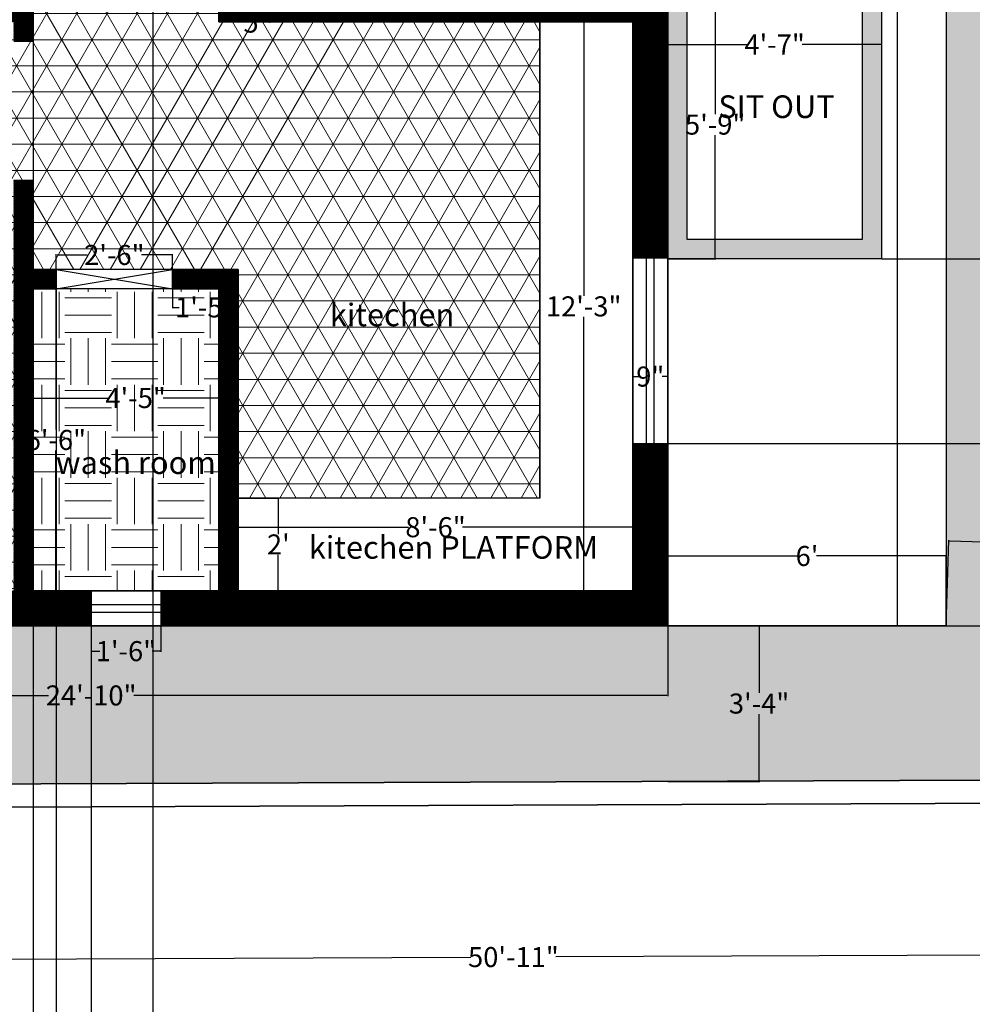
# Model space of a CAD drawing. Units: inches. Extents: x -157 to 1464, y -361 to 1077.
# Tile 4 of 9: x 430 to 676, y 14 to 268. Entities that reach past the tile are written whole.
import ezdxf

# ---------------------------------------------------------------- set-up
doc = ezdxf.new("R2010")
doc.units = ezdxf.units.IN
doc.header["$MEASUREMENT"] = 0
for name, color, linetype, lineweight in [('A-ANNO-DIMS', 2, 'Continuous', 18), ('A-ANNO-TEXT', 7, 'Continuous', 18), ('A-AREA-IDEN', 7, 'Continuous', 18), ('A-FLOR', 7, 'Continuous', 25), ('A-FLOR-FIXT', 9, 'Continuous', 25), ('A-FLOR-PATT', 8, 'Continuous', 13), ('A-WALL', 7, 'Continuous', 35), ('A-WALL-PATT', 252, 'Continuous', 13), ('C-ANNO-DIMS', 2, 'Continuous', 18), ('C-PROP', 7, 'Continuous', 35), ('doors and windows', 33, 'Continuous', 25), ('L-GRND-PATT', 8, 'Continuous', 13)]:
    doc.layers.add(name, color=color, linetype=linetype, lineweight=lineweight)
doc.styles.get("Standard").update_dxf_attribs({"font": 'arial.ttf'})
doc.dimstyles.new('Annotative', dxfattribs={"dimscale": 0, "dimtxt": 5.18, "dimasz": 0.18, "dimexe": 0.18, "dimexo": 0.0625, "dimgap": 0.09, "dimtad": 0, "dimtih": 1, "dimtoh": 1, "dimdec": 0, "dimzin": 0, "dimdsep": 46, "dimlunit": 3, "dimtxsty": 'Standard', "dimcen": 0.09, "dimadec": 0, "dimazin": 0, "dimtfac": 1, "dimtdec": 0, "dimtofl": 0, "dimtmove": 0, "dimatfit": 3, "dimfxl": 1, "dimtolj": 1, "dimtzin": 0, "dimarcsym": 0})

# ---------------------------------------------------------------- blocks, each defined once
blk = doc.blocks.new('*D2')
at = {"layer": 'A-ANNO-DIMS', "color": 0, "lineweight": -2, "transparency": 16777216}
for p, q in [((298.97, 111.8), (298.97, 93.67)), ((596.97, 111.8), (596.97, 93.67)), ((299.15, 93.85), (436.92, 93.85)), ((596.79, 93.85), (459.01, 93.85))]:
    blk.add_line(p, q, dxfattribs=at)
at = {"layer": 'A-ANNO-DIMS', "color": 0, "transparency": 16777216}
for points in [[(299.15, 93.88), (299.15, 93.82), (298.97, 93.85)], [(596.79, 93.88), (596.79, 93.82), (596.97, 93.85)]]:
    blk.add_solid(points, dxfattribs=at)
at = {"layer": 'Defpoints', "color": 0, "transparency": 16777216}
for p in [(298.97, 111.86), (596.97, 111.86), (596.97, 93.85)]:
    blk.add_point(p, dxfattribs=at)
at = {"layer": 'A-ANNO-DIMS', "color": 0, "transparency": 16777216, "insert": (447.97, 93.85), "char_height": 5.18, "attachment_point": 5}
blk.add_mtext('\\A1;24\'-10"', dxfattribs=at)
blk = doc.blocks.new('*D5')
at = {"layer": 'A-ANNO-DIMS', "color": 0, "lineweight": -2, "transparency": 16777216}
for p, q in [((433.03, 198.86), (439.03, 198.86)), ((438.85, 198.68), (438.85, 162.6)), ((438.85, 121.04), (438.85, 157.13)), ((433.03, 120.86), (439.03, 120.86))]:
    blk.add_line(p, q, dxfattribs=at)
at = {"layer": 'A-ANNO-DIMS', "color": 0, "transparency": 16777216}
for points in [[(438.82, 198.68), (438.88, 198.68), (438.85, 198.86)], [(438.82, 121.04), (438.88, 121.04), (438.85, 120.86)]]:
    blk.add_solid(points, dxfattribs=at)
at = {"layer": 'Defpoints', "color": 0, "transparency": 16777216}
for p in [(432.97, 198.86), (438.85, 198.86), (432.97, 120.86)]:
    blk.add_point(p, dxfattribs=at)
at = {"layer": 'A-ANNO-DIMS', "color": 0, "transparency": 16777216, "insert": (438.85, 159.86), "char_height": 5.18, "attachment_point": 5}
blk.add_mtext('\\A1;6\'-6"', dxfattribs=at)
blk = doc.blocks.new('*D6')
at = {"layer": 'A-ANNO-DIMS', "color": 0, "lineweight": -2, "transparency": 16777216}
for p, q in [((432.97, 198.8), (432.97, 170.51)), ((485.97, 198.8), (485.97, 170.51)), ((433.15, 170.69), (452.39, 170.69)), ((485.79, 170.69), (466.55, 170.69))]:
    blk.add_line(p, q, dxfattribs=at)
at = {"layer": 'A-ANNO-DIMS', "color": 0, "transparency": 16777216}
for points in [[(433.15, 170.72), (433.15, 170.66), (432.97, 170.69)], [(485.79, 170.72), (485.79, 170.66), (485.97, 170.69)]]:
    blk.add_solid(points, dxfattribs=at)
at = {"layer": 'Defpoints', "color": 0, "transparency": 16777216}
for p in [(432.97, 198.86), (485.97, 198.86), (485.97, 170.69)]:
    blk.add_point(p, dxfattribs=at)
at = {"layer": 'A-ANNO-DIMS', "color": 0, "transparency": 16777216, "insert": (459.47, 170.69), "char_height": 5.18, "attachment_point": 5}
blk.add_mtext('\\A1;4\'-5"', dxfattribs=at)
blk = doc.blocks.new('*D11')
at = {"layer": 'A-ANNO-DIMS', "color": 0, "lineweight": -2, "transparency": 16777216}
for p, q in [((485.97, 120.92), (485.97, 137.5)), ((587.97, 120.92), (587.97, 137.5)), ((486.15, 137.32), (529.99, 137.32)), ((587.79, 137.32), (543.95, 137.32))]:
    blk.add_line(p, q, dxfattribs=at)
at = {"layer": 'A-ANNO-DIMS', "color": 0, "transparency": 16777216}
for points in [[(486.15, 137.35), (486.15, 137.29), (485.97, 137.32)], [(587.79, 137.35), (587.79, 137.29), (587.97, 137.32)]]:
    blk.add_solid(points, dxfattribs=at)
at = {"layer": 'Defpoints', "color": 0, "transparency": 16777216}
for p in [(485.97, 137.32), (485.97, 120.86), (587.97, 120.86)]:
    blk.add_point(p, dxfattribs=at)
at = {"layer": 'A-ANNO-DIMS', "color": 0, "transparency": 16777216, "insert": (536.97, 137.32), "char_height": 5.18, "attachment_point": 5}
blk.add_mtext('\\A1;8\'-6"', dxfattribs=at)
blk = doc.blocks.new('*D12')
at = {"layer": 'A-ANNO-DIMS', "color": 0, "lineweight": -2, "transparency": 16777216}
for p, q in [((587.9, 267.86), (575.08, 267.86)), ((575.26, 267.68), (575.26, 197.1)), ((575.26, 121.04), (575.26, 191.62)), ((587.9, 120.86), (575.08, 120.86))]:
    blk.add_line(p, q, dxfattribs=at)
at = {"layer": 'A-ANNO-DIMS', "color": 0, "transparency": 16777216}
for points in [[(575.23, 267.68), (575.29, 267.68), (575.26, 267.86)], [(575.23, 121.04), (575.29, 121.04), (575.26, 120.86)]]:
    blk.add_solid(points, dxfattribs=at)
at = {"layer": 'Defpoints', "color": 0, "transparency": 16777216}
for p in [(575.26, 267.86), (587.97, 267.86), (587.97, 120.86)]:
    blk.add_point(p, dxfattribs=at)
at = {"layer": 'A-ANNO-DIMS', "color": 0, "transparency": 16777216, "insert": (575.26, 194.36), "char_height": 5.18, "attachment_point": 5}
blk.add_mtext('\\A1;12\'-3"', dxfattribs=at)
blk = doc.blocks.new('*D14')
at = {"layer": 'C-ANNO-DIMS', "color": 0, "lineweight": -2, "transparency": 16777216}
for p, q in [((862.57, 66.62), (862.72, 27.26)), ((251.33, 64.28), (251.48, 24.92)), ((251.66, 25.1), (546.1, 26.23)), ((862.54, 27.44), (568.1, 26.31))]:
    blk.add_line(p, q, dxfattribs=at)
at = {"layer": 'C-ANNO-DIMS', "color": 0, "transparency": 16777216}
for points in [[(862.54, 27.47), (862.54, 27.41), (862.72, 27.44)], [(251.66, 25.13), (251.66, 25.07), (251.48, 25.1)]]:
    blk.add_solid(points, dxfattribs=at)
at = {"layer": 'Defpoints', "color": 0, "transparency": 16777216}
for p in [(862.57, 66.68), (251.33, 64.34), (862.72, 27.44)]:
    blk.add_point(p, dxfattribs=at)
at = {"layer": 'C-ANNO-DIMS', "color": 0, "transparency": 16777216, "insert": (557.1, 26.27), "char_height": 5.18, "attachment_point": 5}
blk.add_mtext('\\A1;50\'-11"', dxfattribs=at)
blk = doc.blocks.new('*D22')
at = {"layer": 'A-ANNO-DIMS', "color": 0, "lineweight": -2, "transparency": 16777216}
for p, q in [((596.97, 111.92), (596.97, 130.06)), ((597.15, 129.88), (630.48, 129.88)), ((668.79, 129.88), (635.45, 129.88)), ((668.97, 111.92), (668.97, 130.06))]:
    blk.add_line(p, q, dxfattribs=at)
at = {"layer": 'A-ANNO-DIMS', "color": 0, "transparency": 16777216}
for points in [[(597.15, 129.91), (597.15, 129.85), (596.97, 129.88)], [(668.79, 129.91), (668.79, 129.85), (668.97, 129.88)]]:
    blk.add_solid(points, dxfattribs=at)
at = {"layer": 'Defpoints', "color": 0, "transparency": 16777216}
for p in [(596.97, 129.88), (596.97, 111.86), (668.97, 111.86)]:
    blk.add_point(p, dxfattribs=at)
at = {"layer": 'A-ANNO-DIMS', "color": 0, "transparency": 16777216, "insert": (632.97, 129.88), "char_height": 5.18, "attachment_point": 5}
blk.add_mtext("\\A1;6'", dxfattribs=at)
blk = doc.blocks.new('*D23')
at = {"layer": 'A-ANNO-DIMS', "color": 0, "lineweight": -2, "transparency": 16777216}
for p, q in [((668.9, 492.86), (656.18, 492.86)), ((656.36, 492.68), (656.36, 305.1)), ((656.36, 112.04), (656.36, 299.62)), ((668.9, 111.86), (656.18, 111.86))]:
    blk.add_line(p, q, dxfattribs=at)
at = {"layer": 'A-ANNO-DIMS', "color": 0, "transparency": 16777216}
for points in [[(656.33, 492.68), (656.39, 492.68), (656.36, 492.86)], [(656.33, 112.04), (656.39, 112.04), (656.36, 111.86)]]:
    blk.add_solid(points, dxfattribs=at)
at = {"layer": 'Defpoints', "color": 0, "transparency": 16777216}
for p in [(668.97, 492.86), (656.36, 111.86), (668.97, 111.86)]:
    blk.add_point(p, dxfattribs=at)
at = {"layer": 'A-ANNO-DIMS', "color": 0, "transparency": 16777216, "insert": (656.36, 302.36), "char_height": 5.18, "attachment_point": 5}
blk.add_mtext('\\A1;31\'-9"', dxfattribs=at)
blk = doc.blocks.new('*D26')
at = {"layer": 'A-ANNO-DIMS', "color": 0, "lineweight": -2, "transparency": 16777216}
for p, q in [((587.97, 184.35), (587.97, 176.05)), ((596.97, 184.35), (596.97, 176.05)), ((588.15, 176.23), (589.4, 176.23)), ((596.79, 176.23), (595.53, 176.23))]:
    blk.add_line(p, q, dxfattribs=at)
at = {"layer": 'A-ANNO-DIMS', "color": 0, "transparency": 16777216}
for points in [[(588.15, 176.26), (588.15, 176.2), (587.97, 176.23)], [(596.79, 176.26), (596.79, 176.2), (596.97, 176.23)]]:
    blk.add_solid(points, dxfattribs=at)
at = {"layer": 'Defpoints', "color": 0, "transparency": 16777216}
for p in [(587.97, 184.41), (596.97, 184.41), (596.97, 176.23)]:
    blk.add_point(p, dxfattribs=at)
at = {"layer": 'A-ANNO-DIMS', "color": 0, "transparency": 16777216, "insert": (592.47, 176.23), "char_height": 5.18, "attachment_point": 5}
blk.add_mtext('\\A1;9"', dxfattribs=at)
blk = doc.blocks.new('*D27')
at = {"layer": 'A-ANNO-DIMS', "color": 0, "lineweight": -2, "transparency": 16777216}
for p, q in [((486.03, 144.86), (496.52, 144.86)), ((496.34, 144.68), (496.34, 135.55)), ((496.34, 121.04), (496.34, 130.17)), ((486.03, 120.86), (496.52, 120.86))]:
    blk.add_line(p, q, dxfattribs=at)
at = {"layer": 'A-ANNO-DIMS', "color": 0, "transparency": 16777216}
for points in [[(496.31, 144.68), (496.37, 144.68), (496.34, 144.86)], [(496.31, 121.04), (496.37, 121.04), (496.34, 120.86)]]:
    blk.add_solid(points, dxfattribs=at)
at = {"layer": 'Defpoints', "color": 0, "transparency": 16777216}
for p in [(485.97, 144.86), (485.97, 120.86), (496.34, 120.86)]:
    blk.add_point(p, dxfattribs=at)
at = {"layer": 'A-ANNO-DIMS', "color": 0, "transparency": 16777216, "insert": (496.34, 132.86), "char_height": 5.18, "attachment_point": 5}
blk.add_mtext("\\A1;2'", dxfattribs=at)
blk = doc.blocks.new('*D29')
at = {"layer": 'A-ANNO-DIMS', "color": 0, "lineweight": -2, "transparency": 16777216}
for p, q in [((438.97, 203.92), (438.97, 207.83)), ((439.15, 207.65), (446.95, 207.65)), ((468.79, 207.65), (460.99, 207.65)), ((468.97, 203.92), (468.97, 207.83))]:
    blk.add_line(p, q, dxfattribs=at)
at = {"layer": 'A-ANNO-DIMS', "color": 0, "transparency": 16777216}
for points in [[(439.15, 207.68), (439.15, 207.62), (438.97, 207.65)], [(468.79, 207.68), (468.79, 207.62), (468.97, 207.65)]]:
    blk.add_solid(points, dxfattribs=at)
at = {"layer": 'Defpoints', "color": 0, "transparency": 16777216}
for p in [(468.97, 207.65), (438.97, 203.86), (468.97, 203.86)]:
    blk.add_point(p, dxfattribs=at)
at = {"layer": 'A-ANNO-DIMS', "color": 0, "transparency": 16777216, "insert": (453.97, 207.65), "char_height": 5.18, "attachment_point": 5}
blk.add_mtext('\\A1;2\'-6"', dxfattribs=at)
blk = doc.blocks.new('*D35')
at = {"layer": 'A-ANNO-DIMS', "color": 0, "lineweight": -2, "transparency": 16777216}
for p, q in [((447.97, 115.3), (447.97, 105.12)), ((465.97, 115.3), (465.97, 105.12)), ((448.15, 105.3), (450.24, 105.3)), ((465.79, 105.3), (463.7, 105.3))]:
    blk.add_line(p, q, dxfattribs=at)
at = {"layer": 'A-ANNO-DIMS', "color": 0, "transparency": 16777216}
for points in [[(448.15, 105.33), (448.15, 105.27), (447.97, 105.3)], [(465.79, 105.33), (465.79, 105.27), (465.97, 105.3)]]:
    blk.add_solid(points, dxfattribs=at)
at = {"layer": 'Defpoints', "color": 0, "transparency": 16777216}
for p in [(447.97, 115.36), (465.97, 115.36), (465.97, 105.3)]:
    blk.add_point(p, dxfattribs=at)
at = {"layer": 'A-ANNO-DIMS', "color": 0, "transparency": 16777216, "insert": (456.97, 105.3), "char_height": 5.18, "attachment_point": 5}
blk.add_mtext('\\A1;1\'-6"', dxfattribs=at)
blk = doc.blocks.new('*D45')
at = {"layer": 'A-ANNO-DIMS', "color": 0, "lineweight": -2, "transparency": 16777216}
for p, q in [((596.97, 275.94), (596.97, 261.84)), ((652.25, 275.94), (652.25, 261.84)), ((597.15, 262.02), (617.53, 262.02)), ((652.07, 262.02), (631.69, 262.02))]:
    blk.add_line(p, q, dxfattribs=at)
at = {"layer": 'A-ANNO-DIMS', "color": 0, "transparency": 16777216}
for points in [[(597.15, 262.05), (597.15, 261.99), (596.97, 262.02)], [(652.07, 262.05), (652.07, 261.99), (652.25, 262.02)]]:
    blk.add_solid(points, dxfattribs=at)
at = {"layer": 'Defpoints', "color": 0, "transparency": 16777216}
for p in [(596.97, 276), (652.25, 276), (652.25, 262.02)]:
    blk.add_point(p, dxfattribs=at)
at = {"layer": 'A-ANNO-DIMS', "color": 0, "transparency": 16777216, "insert": (624.61, 262.02), "char_height": 5.18, "attachment_point": 5}
blk.add_mtext('\\A1;4\'-7"', dxfattribs=at)
blk = doc.blocks.new('*D46')
at = {"layer": 'A-ANNO-DIMS', "color": 0, "lineweight": -2, "transparency": 16777216}
for p, q in [((597.03, 276), (609.43, 276)), ((609.25, 275.82), (609.25, 244.05)), ((609.25, 206.81), (609.25, 238.58)), ((597.03, 206.63), (609.43, 206.63))]:
    blk.add_line(p, q, dxfattribs=at)
at = {"layer": 'A-ANNO-DIMS', "color": 0, "transparency": 16777216}
for points in [[(609.22, 275.82), (609.28, 275.82), (609.25, 276)], [(609.22, 206.81), (609.28, 206.81), (609.25, 206.63)]]:
    blk.add_solid(points, dxfattribs=at)
at = {"layer": 'Defpoints', "color": 0, "transparency": 16777216}
for p in [(596.97, 276), (609.25, 276), (596.97, 206.63)]:
    blk.add_point(p, dxfattribs=at)
at = {"layer": 'A-ANNO-DIMS', "color": 0, "transparency": 16777216, "insert": (609.25, 241.32), "char_height": 5.18, "attachment_point": 5}
blk.add_mtext('\\A1;5\'-9"', dxfattribs=at)
blk = doc.blocks.new('*D47')
at = {"layer": 'A-ANNO-DIMS', "color": 0, "lineweight": -2, "transparency": 16777216}
for p, q in [((468.97, 203.8), (468.97, 193.92)), ((485.97, 203.8), (485.97, 193.92)), ((469.15, 194.1), (470.74, 194.1)), ((485.79, 194.1), (484.2, 194.1))]:
    blk.add_line(p, q, dxfattribs=at)
at = {"layer": 'A-ANNO-DIMS', "color": 0, "transparency": 16777216}
for points in [[(469.15, 194.13), (469.15, 194.07), (468.97, 194.1)], [(485.79, 194.13), (485.79, 194.07), (485.97, 194.1)]]:
    blk.add_solid(points, dxfattribs=at)
at = {"layer": 'Defpoints', "color": 0, "transparency": 16777216}
for p in [(468.97, 203.86), (485.97, 203.86), (468.97, 194.1)]:
    blk.add_point(p, dxfattribs=at)
at = {"layer": 'A-ANNO-DIMS', "color": 0, "transparency": 16777216, "insert": (477.47, 194.1), "char_height": 5.18, "attachment_point": 5}
blk.add_mtext('\\A1;1\'-5"', dxfattribs=at)
blk = doc.blocks.new('*D48')
at = {"layer": 'A-ANNO-DIMS', "color": 0, "lineweight": -2, "transparency": 16777216}
for p, q in [((481.03, 272.86), (494.39, 272.86)), ((494.21, 272.68), (494.21, 268.04)), ((481.03, 267.86), (494.39, 267.86)), ((494.21, 267.68), (494.03, 267.68)), ((494.21, 267.86), (494.21, 267.68))]:
    blk.add_line(p, q, dxfattribs=at)
at = {"layer": 'A-ANNO-DIMS', "color": 0, "transparency": 16777216}
for points in [[(494.18, 272.68), (494.24, 272.68), (494.21, 272.86)], [(494.18, 268.04), (494.24, 268.04), (494.21, 267.86)]]:
    blk.add_solid(points, dxfattribs=at)
at = {"layer": 'Defpoints', "color": 0, "transparency": 16777216}
for p in [(480.97, 272.86), (480.97, 267.86), (494.21, 267.86)]:
    blk.add_point(p, dxfattribs=at)
at = {"layer": 'A-ANNO-DIMS', "color": 0, "transparency": 16777216, "insert": (490.96, 267.68), "char_height": 5.18, "attachment_point": 5}
blk.add_mtext('\\A1;5"', dxfattribs=at)
blk = doc.blocks.new('*D55')
at = {"layer": 'C-ANNO-DIMS', "color": 0, "lineweight": -2, "transparency": 16777216}
for p, q in [((597.03, 111.86), (620.77, 111.86)), ((620.59, 111.68), (620.59, 94.5)), ((620.59, 71.84), (620.59, 89.03)), ((597.03, 71.66), (620.77, 71.66))]:
    blk.add_line(p, q, dxfattribs=at)
at = {"layer": 'C-ANNO-DIMS', "color": 0, "transparency": 16777216}
for points in [[(620.56, 111.68), (620.62, 111.68), (620.59, 111.86)], [(620.56, 71.84), (620.62, 71.84), (620.59, 71.66)]]:
    blk.add_solid(points, dxfattribs=at)
at = {"layer": 'Defpoints', "color": 0, "transparency": 16777216}
for p in [(596.97, 111.86), (596.97, 71.66), (620.59, 71.66)]:
    blk.add_point(p, dxfattribs=at)
at = {"layer": 'C-ANNO-DIMS', "color": 0, "transparency": 16777216, "insert": (620.59, 91.76), "char_height": 5.18, "attachment_point": 5}
blk.add_mtext('\\A1;3\'-4"', dxfattribs=at)
blk = doc.blocks.new('*D56')
at = {"layer": 'C-ANNO-DIMS', "color": 0, "lineweight": -2, "transparency": 16777216}
for p, q in [((668.97, 111.92), (669.64, 133.96)), ((669.82, 133.77), (754.7, 131.17)), ((857.06, 128.03), (772.18, 130.63)), ((856.57, 106.17), (857.25, 128.21))]:
    blk.add_line(p, q, dxfattribs=at)
at = {"layer": 'C-ANNO-DIMS', "color": 0, "transparency": 16777216}
for points in [[(669.82, 133.8), (669.82, 133.74), (669.64, 133.78)], [(857.06, 128.06), (857.06, 128), (857.24, 128.03)]]:
    blk.add_solid(points, dxfattribs=at)
at = {"layer": 'Defpoints', "color": 0, "transparency": 16777216}
for p in [(857.24, 128.03), (668.97, 111.86), (856.57, 106.11)]:
    blk.add_point(p, dxfattribs=at)
at = {"layer": 'C-ANNO-DIMS', "color": 0, "transparency": 16777216, "insert": (763.44, 130.9), "char_height": 5.18, "attachment_point": 5}
blk.add_mtext('\\A1;15\'-8"', dxfattribs=at)
blk = doc.blocks.new('WIN-48x9')
for p, q in [((9, 48), (0, 48)), ((0, 48), (0, 0)), ((3.5, 48), (3.5, 0)), ((5.5, 48), (5.5, 0)), ((9, 48), (9, 0)), ((9, 0), (0, 0))]:
    blk.add_line(p, q)
blk = doc.blocks.new('*D73')
at = {"layer": 'A-ANNO-DIMS', "color": 0, "lineweight": -2, "transparency": 16777216}
for p, q in [((432.97, 411.8), (432.97, -357.73)), ((463.95, 411.8), (463.95, -357.73)), ((433.15, -357.55), (441.44, -357.55)), ((463.77, -357.55), (455.48, -357.55))]:
    blk.add_line(p, q, dxfattribs=at)
at = {"layer": 'A-ANNO-DIMS', "color": 0, "transparency": 16777216}
for points in [[(433.15, -357.52), (433.15, -357.58), (432.97, -357.55)], [(463.77, -357.52), (463.77, -357.58), (463.95, -357.55)]]:
    blk.add_solid(points, dxfattribs=at)
at = {"layer": 'Defpoints', "color": 0, "transparency": 16777216}
for p in [(432.97, 411.86), (463.95, 411.86), (463.95, -357.55)]:
    blk.add_point(p, dxfattribs=at)
at = {"layer": 'A-ANNO-DIMS', "color": 0, "transparency": 16777216, "insert": (448.46, -357.55), "char_height": 5.18, "attachment_point": 5}
blk.add_mtext('\\A1;2\'-7"', dxfattribs=at)
blk = doc.blocks.new('*D74')
at = {"layer": 'A-ANNO-DIMS', "color": 0, "lineweight": -2, "transparency": 16777216}
for p, q in [((597.03, 158.9), (1397.57, 158.9)), ((1397.39, 158.72), (1397.39, 138.11)), ((1397.39, 112.04), (1397.39, 132.64)), ((597.03, 111.86), (1397.57, 111.86))]:
    blk.add_line(p, q, dxfattribs=at)
at = {"layer": 'A-ANNO-DIMS', "color": 0, "transparency": 16777216}
for points in [[(1397.36, 158.72), (1397.42, 158.72), (1397.39, 158.9)], [(1397.36, 112.04), (1397.42, 112.04), (1397.39, 111.86)]]:
    blk.add_solid(points, dxfattribs=at)
at = {"layer": 'Defpoints', "color": 0, "transparency": 16777216}
for p in [(596.97, 158.9), (1397.39, 158.9), (596.97, 111.86)]:
    blk.add_point(p, dxfattribs=at)
at = {"layer": 'A-ANNO-DIMS', "color": 0, "transparency": 16777216, "insert": (1397.39, 135.38), "char_height": 5.18, "attachment_point": 5}
blk.add_mtext('\\A1;3\'-11"', dxfattribs=at)
blk = doc.blocks.new('*D75')
at = {"layer": 'A-ANNO-DIMS', "color": 0, "lineweight": -2, "transparency": 16777216}
for p, q in [((432.97, 120.8), (432.97, -357.73)), ((447.97, 120.8), (447.97, -357.73)), ((433.15, -357.55), (433.74, -357.55)), ((447.79, -357.55), (447.2, -357.55))]:
    blk.add_line(p, q, dxfattribs=at)
at = {"layer": 'A-ANNO-DIMS', "color": 0, "transparency": 16777216}
for points in [[(433.15, -357.52), (433.15, -357.58), (432.97, -357.55)], [(447.79, -357.52), (447.79, -357.58), (447.97, -357.55)]]:
    blk.add_solid(points, dxfattribs=at)
at = {"layer": 'Defpoints', "color": 0, "transparency": 16777216}
for p in [(432.97, 120.86), (447.97, 120.86), (447.97, -357.55)]:
    blk.add_point(p, dxfattribs=at)
at = {"layer": 'A-ANNO-DIMS', "color": 0, "transparency": 16777216, "insert": (440.47, -357.55), "char_height": 5.18, "attachment_point": 5}
blk.add_mtext('\\A1;1\'-3"', dxfattribs=at)
blk = doc.blocks.new('*D79')
at = {"layer": 'A-ANNO-DIMS', "color": 0, "lineweight": -2, "transparency": 16777216}
for p, q in [((438.97, 203.8), (438.97, -357.73)), ((432.97, 198.8), (432.97, -357.73)), ((433.15, -357.55), (438.79, -357.55)), ((438.97, -357.55), (439.15, -357.55))]:
    blk.add_line(p, q, dxfattribs=at)
at = {"layer": 'A-ANNO-DIMS', "color": 0, "transparency": 16777216}
for points in [[(433.15, -357.52), (433.15, -357.58), (432.97, -357.55)], [(438.79, -357.52), (438.79, -357.58), (438.97, -357.55)]]:
    blk.add_solid(points, dxfattribs=at)
at = {"layer": 'Defpoints', "color": 0, "transparency": 16777216}
for p in [(438.97, 203.86), (432.97, 198.86), (438.97, -357.55)]:
    blk.add_point(p, dxfattribs=at)
at = {"layer": 'A-ANNO-DIMS', "color": 0, "transparency": 16777216, "insert": (446.12, -357.55), "char_height": 5.18, "attachment_point": 5}
blk.add_mtext('\\A1;0\'-6"', dxfattribs=at)
blk = doc.blocks.new('*D81')
at = {"layer": 'A-ANNO-DIMS', "color": 0, "lineweight": -2, "transparency": 16777216}
for p, q in [((563.97, 144.92), (563.97, 1069.66)), ((564.15, 1069.48), (568.95, 1069.48)), ((587.79, 1069.48), (582.99, 1069.48)), ((587.97, 120.92), (587.97, 1069.66))]:
    blk.add_line(p, q, dxfattribs=at)
at = {"layer": 'A-ANNO-DIMS', "color": 0, "transparency": 16777216}
for points in [[(564.15, 1069.51), (564.15, 1069.45), (563.97, 1069.48)], [(587.79, 1069.51), (587.79, 1069.45), (587.97, 1069.48)]]:
    blk.add_solid(points, dxfattribs=at)
at = {"layer": 'Defpoints', "color": 0, "transparency": 16777216}
for p in [(587.97, 1069.48), (563.97, 144.86), (587.97, 120.86)]:
    blk.add_point(p, dxfattribs=at)
at = {"layer": 'A-ANNO-DIMS', "color": 0, "transparency": 16777216, "insert": (575.97, 1069.48), "char_height": 5.18, "attachment_point": 5}
blk.add_mtext('\\A1;2\'-0"', dxfattribs=at)
blk = doc.blocks.new('*D83')
at = {"layer": 'A-ANNO-DIMS', "color": 0, "lineweight": -2, "transparency": 16777216}
for p, q in [((652.31, 206.63), (1397.57, 206.63)), ((1397.39, 206.45), (1397.39, 161.94)), ((1397.39, 112.04), (1397.39, 156.56)), ((597.03, 111.86), (1397.57, 111.86))]:
    blk.add_line(p, q, dxfattribs=at)
at = {"layer": 'A-ANNO-DIMS', "color": 0, "transparency": 16777216}
for points in [[(1397.36, 206.45), (1397.42, 206.45), (1397.39, 206.63)], [(1397.36, 112.04), (1397.42, 112.04), (1397.39, 111.86)]]:
    blk.add_solid(points, dxfattribs=at)
at = {"layer": 'Defpoints', "color": 0, "transparency": 16777216}
for p in [(652.25, 206.63), (1397.39, 206.63), (596.97, 111.86)]:
    blk.add_point(p, dxfattribs=at)
at = {"layer": 'A-ANNO-DIMS', "color": 0, "transparency": 16777216, "insert": (1397.39, 159.25), "char_height": 5.18, "attachment_point": 5}
blk.add_mtext('\\A1;7\'-11"', dxfattribs=at)

msp = doc.modelspace()

# ---------------------------------------------------------------- hatches: boundary and pattern name
at = {"layer": 'A-FLOR-PATT'}
h = msp.add_hatch(color=256, dxfattribs=at)
h.dxf.hatch_style = 1
h.paths.add_polyline_path([(652.25, 276), (596.97, 276), (596.97, 206.63), (652.25, 206.63)])
h.paths.add_polyline_path([(647.25, 271), (647.25, 211.63), (601.97, 211.63), (601.97, 271)], flags=16)
h = msp.add_hatch(dxfattribs=at)
h.set_pattern_fill('NET3', color=256, scale=54)
h.paths.add_polyline_path([(563.97, 267.86), (480.97, 267.86), (480.97, 272.86), (432.97, 272.86), (432.97, 262.86), (427.97, 262.86), (427.97, 267.86), (307.97, 267.86), (307.97, 120.86), (427.97, 120.86), (427.97, 226.86), (432.97, 226.86), (432.97, 203.86), (438.97, 203.86), (468.97, 203.86), (485.97, 203.86), (485.97, 144.86), (563.97, 144.86)])
h.paths.add_polyline_path([(507.66, 186.06), (540.97, 186.06), (540.97, 198.1), (507.66, 198.1)], flags=24)
h.paths.add_polyline_path([(343.4, 209.88), (389.84, 209.88), (389.84, 221.92), (343.4, 221.92)], flags=24)
h = msp.add_hatch(dxfattribs=at)
h.set_pattern_fill('EARTH', color=256, scale=48)
h.set_pattern_definition([(0, (213.194, 103.601), (12, 12), [12, -12]), (0, (213.194, 108.101), (12, 12), [12, -12]), (0, (213.194, 112.601), (12, 12), [12, -12]), (90, (214.694, 114.101), (-12, 12), [12, -12]), (90, (219.194, 114.101), (-12, 12), [12, -12]), (90, (223.694, 114.101), (-12, 12), [12, -12])])
h.paths.add_polyline_path([(480.97, 198.86), (468.97, 198.86), (438.97, 198.86), (432.97, 198.86), (432.97, 120.86), (480.97, 120.86)])
at = {"layer": 'A-WALL-PATT'}
h = msp.add_hatch(dxfattribs=at)
h.set_pattern_fill('ANSI31', color=256)
h.set_pattern_definition([(45, (213.19381, 103.60139), (-0.088388348, 0.088388348), [])])
h.paths.add_polyline_path([(307.97, 267.86), (427.97, 267.86), (427.97, 262.86), (432.97, 262.86), (432.97, 277.86), (427.97, 277.86), (427.97, 272.86), (307.97, 272.86), (307.97, 276.53), (298.97, 276.53), (298.97, 194.36), (307.97, 194.36)])
h.paths.add_polyline_path([(307.97, 411.86), (427.97, 411.86), (427.97, 313.86), (432.97, 313.86), (432.97, 411.86), (463.95, 411.86), (463.95, 420.86), (298.97, 420.86), (298.97, 324.53), (307.97, 324.53)])
h.paths.add_polyline_path([(511.95, 420.86), (511.95, 411.86), (546.97, 411.86), (546.97, 420.86)])
h.paths.add_polyline_path([(587.97, 411.86), (587.97, 405.86), (596.97, 405.86), (596.97, 420.86), (582.97, 420.86), (582.97, 411.86)])
h.paths.add_polyline_path([(587.97, 369.86), (587.97, 324), (596.97, 324), (596.97, 369.86)])
h.paths.add_polyline_path([(596.97, 276), (587.97, 276), (587.97, 272.86), (480.97, 272.86), (480.97, 267.86), (587.97, 267.86), (587.97, 206.9), (596.97, 206.9)])
h.paths.add_polyline_path([(587.97, 120.86), (485.97, 120.86), (485.97, 203.86), (468.97, 203.86), (468.97, 198.86), (480.97, 198.86), (480.97, 120.86), (465.97, 120.86), (465.97, 111.86), (596.97, 111.86), (596.97, 158.9), (587.97, 158.9)])
h.paths.add_polyline_path([(427.97, 120.86), (307.97, 120.86), (307.97, 146.36), (298.97, 146.36), (298.97, 111.86), (447.97, 111.86), (447.97, 120.86), (432.97, 120.86), (432.97, 198.86), (438.97, 198.86), (438.97, 203.86), (432.97, 203.86), (432.97, 226.86), (427.97, 226.86)])
at = {"layer": 'L-GRND-PATT'}
h = msp.add_hatch(dxfattribs=at)
h.set_pattern_fill('GRAVEL', color=256, scale=26)
h.set_pattern_definition([(228.01279, (18.72, 26), (-208, -234), [3.49794, -346.2963]), (184.96974, (16.38, 23.4), (312, 26), [6.00257, -594.25404]), (132.51045, (10.4, 22.88), (260, -286), [4.2325, -419.01685]), (267.27369, (0.26, 16.38), (26, 520), [5.4662, -541.1525]), (292.83365, (0, 10.92), (-130, 312), [5.36003, -530.6437]), (357.27369, (2.08, 5.98), (-520, 26), [5.4662, -541.1525]), (37.69424, (7.54, 5.72), (-338, -260), [7.22875, -715.64606]), (72.25533, (13.26, 10.14), (182, 572), [6.8247, -675.64436]), (121.42957, (15.34, 16.64), (-208, 338), [5.4847, -542.9859]), (175.23636, (12.48, 21.32), (286, -26), [6.26163, -306.81983]), (222.39744, (6.24, 21.84), (-312, -286), [8.09765, -801.66775]), (138.81407, (26, 16.12), (-182, 156), [2.76383, -273.61997]), (171.46923, (23.92, 17.94), (338, -52), [5.25816, -520.5593]), (225, (18.72, 18.72), (-3e-15, -26), [3.67695, -33.0926]), (203.1986, (16.9, 21.84), (130, 52), [1.9801, -196.03]), (291.8014, (15.08, 21.06), (-26, 78), [2.8003, -137.214]), (30.96376, (16.12, 18.46), (78, 52), [4.54815, -147.0566]), (161.56505, (20.02, 20.8), (52, -26), [3.28877, -78.93045]), (16.38954, (0, 21.06), (260, 78), [4.6072, -456.11397]), (70.34618, (4.42, 22.36), (-104, -286), [3.8652, -382.6526]), (293.1986, (20.02, 26), (-52, 130), [3.9602, -194.0499]), (343.61046, (21.58, 22.36), (-260, 78), [4.6072, -456.11397]), (339.44395, (0, 4.94), (-130, 52), [4.4429, -217.7012]), (294.77514, (4.16, 3.38), (-130, 286), [3.72263, -368.5407]), (66.8014, (20.28, 0), (52, 130), [3.9602, -194.0499]), (17.35402, (21.84, 3.64), (-338, -104), [4.3584, -431.481]), (69.44395, (7.54, 0), (-52, -130), [2.22144, -219.92266]), (101.30993, (18.72, 0), (-26, 104), [1.32574, -131.24877]), (165.96376, (18.46, 1.3), (78, -26), [5.36003, -101.8407]), (186.009, (13.26, 2.6), (260, 26), [4.9673, -491.762]), (303.6901, (16.12, 16.12), (-26, 52), [3.7498, -89.99456]), (353.15723, (18.2, 13), (442, -52), [6.54664, -648.11663]), (60.9454, (24.7, 12.22), (-104, -182), [2.67686, -265.00953]), (90, (26, 14.56), (-26, 26), [1.56, -24.44]), (120.25644, (12.74, 3.38), (104, -182), [3.61202, -357.5915]), (48.01279, (10.92, 6.5), (208, 234), [6.99587, -342.79835]), (0, (15.6, 11.7), (26, 26), [6.76, -19.24]), (325.30485, (22.36, 11.7), (260, -182), [4.11096, -406.98513]), (254.0546, (25.74, 9.36), (-26, -104), [3.78565, -185.4972]), (207.64598, (24.7, 5.72), (-494, -260), [6.1637, -610.20633]), (175.42608, (19.24, 2.86), (-338, 26), [6.52077, -645.5559])])
h.paths.add_polyline_path([(856.57, 645.71), (257.33, 643.42), (257.33, 70.37), (856.57, 72.66)])
h.paths.add_polyline_path([(668.97, 111.86), (596.97, 111.86), (298.97, 111.86), (298.97, 420.86), (298.97, 492.86), (427.97, 492.86), (668.97, 492.86)], flags=16)
h.paths.add_polyline_path([(842.44, 305.24), (842.44, 199.78), (692.18, 199.78), (692.18, 305.24)], flags=16)
h.paths.add_polyline_path([(596.97, 369.86), (596.97, 158.9), (587.97, 158.9), (587.97, 120.86), (485.97, 120.86), (485.97, 203.86), (468.97, 203.86), (468.97, 198.86), (480.97, 198.86), (480.97, 120.86), (465.97, 120.86), (465.97, 111.86), (447.97, 111.86), (447.97, 120.86), (432.97, 120.86), (432.97, 198.86), (438.97, 198.86), (438.97, 203.86), (432.97, 203.86), (432.97, 226.86), (427.97, 226.86), (427.97, 120.86), (307.97, 120.86), (307.97, 146.36), (298.97, 146.36), (298.97, 194.36), (307.97, 194.36), (307.97, 267.86), (427.97, 267.86), (427.97, 262.86), (432.97, 262.86), (432.97, 277.86), (427.97, 277.86), (427.97, 272.86), (307.97, 272.86), (307.97, 276.53), (298.97, 276.53), (298.97, 324.53), (307.97, 324.53), (307.97, 411.86), (427.97, 411.86), (427.97, 313.86), (432.97, 313.86), (432.97, 411.86), (463.95, 411.86), (463.95, 420.86), (334.97, 420.86), (334.97, 456.86), (427.97, 456.86), (427.97, 420.86), (546.97, 420.86), (582.97, 420.86), (596.97, 420.86), (596.97, 405.86)], flags=0)
h.paths.add_polyline_path([(596.97, 369.86), (587.97, 369.86), (587.97, 324), (596.97, 324), (596.97, 276), (587.97, 276), (587.97, 369.86), (587.97, 405.86), (587.97, 411.86), (582.97, 411.86), (546.97, 411.86), (546.97, 420.86), (564.97, 416.36), (582.97, 420.86), (582.97, 411.86), (587.97, 411.86), (587.97, 405.86), (596.97, 405.86), (592.47, 387.86)], flags=0)
h.paths.add_polyline_path([(468.97, 203.86), (468.97, 198.86), (438.97, 198.86), (438.97, 203.86)], flags=0)
h.paths.add_polyline_path([(267.35, 260.99), (288.37, 260.99), (288.37, 271.66), (267.35, 271.66)], flags=24)
h.paths.add_polyline_path([(435.51, 88.48), (460.55, 88.48), (460.55, 99.15), (435.51, 99.15)], flags=24)
h.paths.add_polyline_path([(315.69, 188.99), (336.72, 188.99), (336.72, 199.66), (315.69, 199.66)], flags=8)
h.paths.add_polyline_path([(361.73, 141.9), (373.75, 141.9), (373.75, 152.57), (361.73, 152.57)], flags=8)
h.paths.add_polyline_path([(430.38, 154.49), (447.38, 154.49), (447.38, 165.16), (430.38, 165.16)], flags=8)
h.paths.add_polyline_path([(451.09, 165.32), (468.09, 165.32), (468.09, 175.99), (451.09, 175.99)], flags=8)
h.paths.add_polyline_path([(361.73, 305.06), (373.75, 305.06), (373.75, 315.74), (361.73, 315.74)], flags=8)
h.paths.add_polyline_path([(316.13, 336.94), (337.15, 336.94), (337.15, 347.62), (316.13, 347.62)], flags=8)
h.paths.add_polyline_path([(484.07, 423.56), (492.07, 423.56), (492.07, 434.24), (484.07, 434.24)], flags=8)
h.paths.add_polyline_path([(560.99, 428.52), (568.98, 428.52), (568.98, 439.19), (560.99, 439.19)], flags=8)
h.paths.add_polyline_path([(528.49, 131.95), (545.49, 131.95), (545.49, 142.62), (528.49, 142.62)], flags=8)
h.paths.add_polyline_path([(564.53, 188.99), (585.55, 188.99), (585.55, 199.66), (564.53, 199.66)], flags=8)

# ---------------------------------------------------------------- linework, layer by layer
at = {"layer": 'A-FLOR'}
for p, q in [((668.97, 492.86), (668.97, 111.86)), ((668.97, 111.86), (596.97, 111.86))]:
    msp.add_line(p, q, dxfattribs=at)
for points in [[(596.97, 276), (652.25, 276), (652.25, 206.63), (596.97, 206.63)], [(601.97, 271), (647.25, 271), (647.25, 211.63), (601.97, 211.63)]]:
    msp.add_lwpolyline(points, close=True, dxfattribs=at)
at = {"layer": 'A-FLOR-FIXT'}
for p, q in [((563.97, 267.86), (563.97, 144.86)), ((563.97, 144.86), (485.97, 144.86))]:
    msp.add_line(p, q, dxfattribs=at)
at = {"layer": 'A-WALL'}
for p, q in [((596.97, 369.86), (596.97, 111.86)), ((432.97, 262.86), (432.97, 277.86)), ((480.97, 267.86), (480.97, 272.86)), ((480.97, 267.86), (587.97, 267.86)), ((587.97, 267.86), (587.97, 120.86)), ((427.97, 262.86), (432.97, 262.86)), ((427.97, 226.86), (432.97, 226.86)), ((432.97, 203.86), (432.97, 226.86)), ((438.97, 203.86), (432.97, 203.86)), ((438.97, 198.86), (438.97, 203.86)), ((485.97, 203.86), (468.97, 203.86)), ((468.97, 198.86), (468.97, 203.86)), ((485.97, 120.86), (485.97, 203.86)), ((432.97, 120.86), (432.97, 198.86)), ((438.97, 198.86), (432.97, 198.86)), ((480.97, 198.86), (468.97, 198.86)), ((480.97, 120.86), (480.97, 198.86)), ((480.97, 120.86), (432.97, 120.86)), ((587.97, 120.86), (485.97, 120.86)), ((596.97, 111.86), (298.97, 111.86))]:
    msp.add_line(p, q, dxfattribs=at)
at = {"layer": 'C-PROP'}
msp.add_lwpolyline([(862.57, 615.42), (862.57, 651.74), (251.33, 649.4), (251.33, 64.34), (862.57, 66.68), (862.57, 519.42)], dxfattribs=at)
msp.add_lwpolyline([(257.33, 70.37), (856.57, 72.66), (856.57, 645.71), (257.33, 643.42)], close=True, dxfattribs=at)
at = {"layer": 'doors and windows'}
for p, q in [((438.97, 198.86), (438.97, 203.86)), ((438.97, 203.86), (468.97, 198.86)), ((438.97, 198.86), (468.97, 203.86)), ((468.97, 203.86), (438.97, 203.86)), ((468.97, 198.86), (468.97, 203.86)), ((468.97, 198.86), (438.97, 198.86)), ((447.97, 120.86), (447.97, 111.86)), ((447.97, 120.86), (465.97, 120.86)), ((465.97, 120.86), (465.97, 111.86)), ((447.97, 117.36), (465.97, 117.36)), ((447.97, 115.36), (465.97, 115.36)), ((447.97, 111.86), (465.97, 111.86))]:
    msp.add_line(p, q, dxfattribs=at)

# ---------------------------------------------------------------- block references
at = {"layer": 'doors and windows', "rotation": 180}
msp.add_blockref('WIN-48x9', (596.97, 206.9), dxfattribs=at)

# ---------------------------------------------------------------- texts
at = {"layer": 'A-ANNO-TEXT', "insert": (504.22, 135.02), "char_height": 5.8395, "attachment_point": 1}
msp.add_mtext_dynamic_manual_height_columns('kitechen PLATFORM', width=87.358, gutter_width=29.2, heights=[13.12], dxfattribs=at)
at = {"layer": 'A-AREA-IDEN', "char_height": 5.84, "attachment_point": 1}
for s, insert in [('SIT OUT', (610.06, 248.87)), ('kitechen', (509.66, 195.09)), ('wash room', (438.85, 156.91))]:
    msp.add_mtext_dynamic_manual_height_columns(s, width=87.358, gutter_width=29.2, heights=[13.12], dxfattribs=dict(at, insert=insert))

# ---------------------------------------------------------------- dimensions: what is measured, and where the dimension line sits
at = {"layer": 'A-ANNO-DIMS'}
for base, p1, p2, override, picture, middle in [((587.97, 1069.48), (563.97, 144.86), (587.97, 120.86), {"dimscale": 1, "dimdec": 1, "dimzin": 1, "dimlunit": 4, "dimfrac": 2}, '*D81', (575.97, 1069.48)), ((463.95, -357.55), (432.97, 411.86), (463.95, 411.86), {"dimscale": 1, "dimdec": 1, "dimzin": 1, "dimlunit": 4, "dimfrac": 2}, '*D73', (448.46, -357.55)), ((652.25, 262.02), (596.97, 276), (652.25, 276), {"dimclrd": 0, "dimclre": 0, "dimclrt": 0}, '*D45', (624.61, 262.02)), ((468.97, 207.65), (438.97, 203.86), (468.97, 203.86), {"dimclrd": 0, "dimclre": 0, "dimclrt": 0}, '*D29', (453.97, 207.65)), ((438.97, -357.55), (432.97, 198.86), (438.97, 203.86), {"dimscale": 1, "dimdec": 1, "dimzin": 1, "dimlunit": 4, "dimfrac": 2}, '*D79', (446.12, -357.55)), ((468.97, 194.1), (485.97, 203.86), (468.97, 203.86), {"dimclrd": 0, "dimclre": 0, "dimclrt": 0}, '*D47', (477.47, 194.1)), ((485.97, 170.69), (432.97, 198.86), (485.97, 198.86), {"dimclrd": 0, "dimclre": 0, "dimclrt": 0}, '*D6', (459.47, 170.69)), ((596.97, 176.23), (587.97, 184.41), (596.97, 184.41), {"dimclrd": 0, "dimclre": 0, "dimclrt": 0}, '*D26', (592.47, 176.23)), ((485.97, 137.32), (587.97, 120.86), (485.97, 120.86), {"dimclrd": 0, "dimclre": 0, "dimclrt": 0}, '*D11', (536.97, 137.32)), ((447.97, -357.55), (432.97, 120.86), (447.97, 120.86), {"dimscale": 1, "dimdec": 1, "dimzin": 1, "dimlunit": 4, "dimfrac": 2}, '*D75', (440.47, -357.55)), ((465.97, 105.3), (447.97, 115.36), (465.97, 115.36), {"dimclrd": 0, "dimclre": 0, "dimclrt": 0}, '*D35', (456.97, 105.3)), ((596.97, 93.85), (298.97, 111.86), (596.97, 111.86), {"dimclrd": 0, "dimclre": 0, "dimclrt": 0}, '*D2', (447.97, 93.85))]:
    dim = msp.add_linear_dim(base=base, p1=p1, p2=p2, dimstyle='Annotative', override=override, dxfattribs=at)
    dim.commit()
    dim.dimension.update_dxf_attribs({"geometry": picture, "text_midpoint": middle})
for base, p1, p2, override, picture, middle in [((656.36, 111.86), (668.97, 492.86), (668.97, 111.86), {"dimclrd": 0, "dimclre": 0, "dimclrt": 0}, '*D23', (656.36, 302.36)), ((609.25, 276), (596.97, 206.63), (596.97, 276), {"dimclrd": 0, "dimclre": 0, "dimclrt": 0}, '*D46', (609.25, 241.32)), ((494.21, 267.86), (480.97, 272.86), (480.97, 267.86), {"dimclrd": 0, "dimclre": 0, "dimclrt": 0}, '*D48', (490.96, 267.68)), ((575.26, 267.86), (587.97, 120.86), (587.97, 267.86), {"dimclrd": 0, "dimclre": 0, "dimclrt": 0}, '*D12', (575.26, 194.36)), ((1397.39, 206.63), (596.97, 111.86), (652.25, 206.63), {"dimscale": 1, "dimdec": 1, "dimzin": 1, "dimlunit": 4, "dimfrac": 2}, '*D83', (1397.39, 159.25)), ((438.85, 198.86), (432.97, 120.86), (432.97, 198.86), {"dimclrd": 0, "dimclre": 0, "dimclrt": 0}, '*D5', (438.85, 159.86)), ((1397.39, 158.9), (596.97, 111.86), (596.97, 158.9), {"dimscale": 1, "dimdec": 1, "dimzin": 1, "dimlunit": 4, "dimfrac": 2}, '*D74', (1397.39, 135.38)), ((496.34, 120.86), (485.97, 144.86), (485.97, 120.86), {"dimclrd": 0, "dimclre": 0, "dimclrt": 0}, '*D27', (496.34, 132.86))]:
    dim = msp.add_linear_dim(base=base, p1=p1, p2=p2, angle=90, dimstyle='Annotative', override=override, dxfattribs=at)
    dim.commit()
    dim.dimension.update_dxf_attribs({"geometry": picture, "text_midpoint": middle})
dim = msp.add_linear_dim(base=(596.97, 129.88), p1=(668.97, 111.86), p2=(596.97, 111.86), dimstyle='Annotative', override={"dimclrd": 0, "dimclre": 0, "dimclrt": 0}, dxfattribs=at)
dim.commit()
dim.dimension.update_dxf_attribs({"geometry": '*D22', "text_midpoint": (632.97, 129.88), "dimtype": 160})
at = {"layer": 'C-ANNO-DIMS'}
for p1, p2, distance, picture, middle in [((668.97, 111.86), (856.57, 106.11), 21.93, '*D56', (763.44, 130.9)), ((251.33, 64.34), (862.57, 66.68), -39.24, '*D14', (557.1, 26.27))]:
    dim = msp.add_aligned_dim(p1=p1, p2=p2, distance=distance, dimstyle='Annotative', override={"dimclrd": 0, "dimclre": 0, "dimclrt": 0}, dxfattribs=at)
    dim.commit()
    dim.dimension.update_dxf_attribs({"geometry": picture, "text_midpoint": middle})
dim = msp.add_linear_dim(base=(620.59, 71.66), p1=(596.97, 111.86), p2=(596.97, 71.66), angle=90, dimstyle='Annotative', override={"dimclrd": 0, "dimclre": 0, "dimclrt": 0}, dxfattribs=at)
dim.commit()
dim.dimension.update_dxf_attribs({"geometry": '*D55', "text_midpoint": (620.59, 91.76)})

doc.saveas('drawing.dxf')
